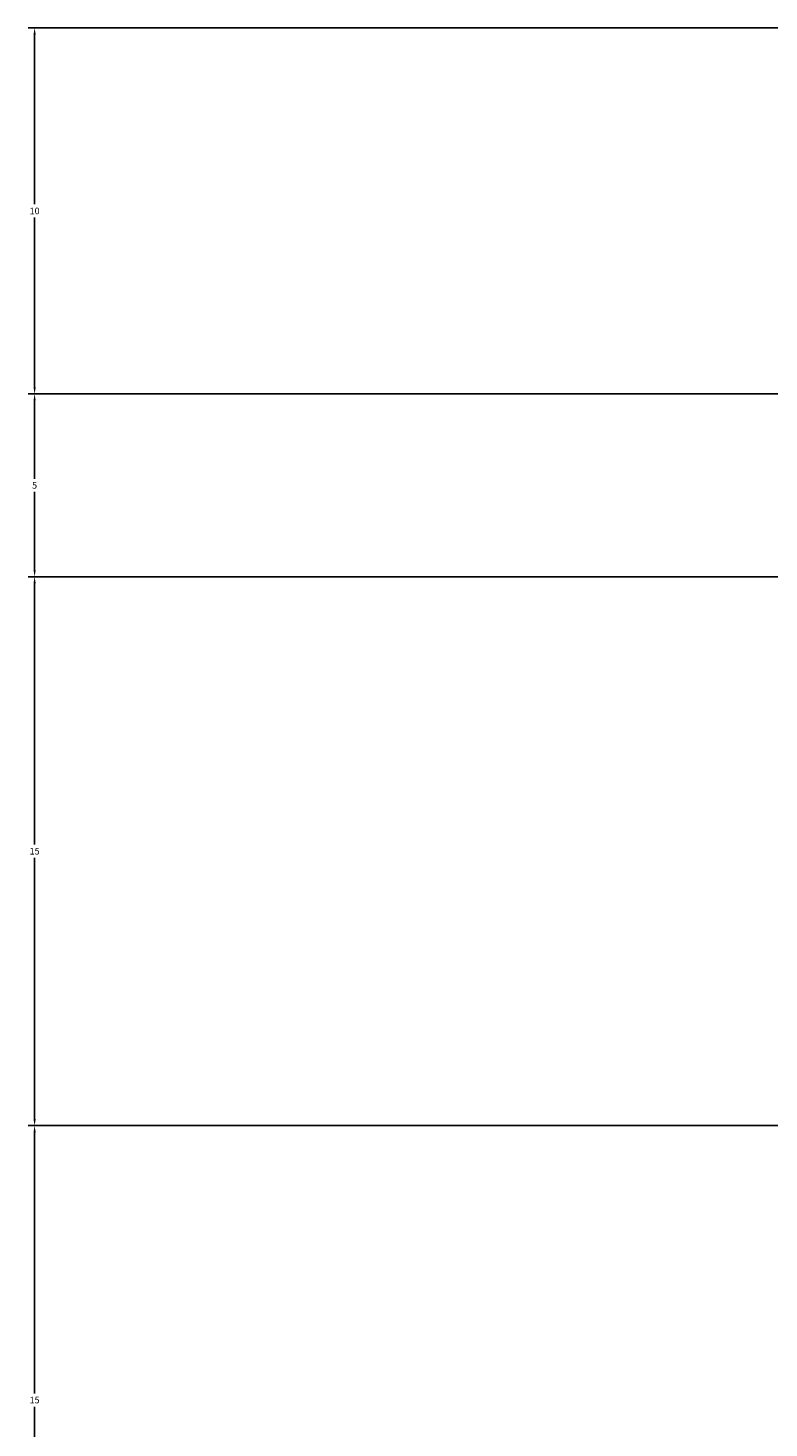
# Model space of a CAD drawing. Units: millimetres. Extents: x -48 to 129, y -118 to -41.
# Tile 2 of 6: x -48 to -28, y -88 to -49. Entities that reach past the tile are written whole.
import ezdxf

# ---------------------------------------------------------------- set-up
doc = ezdxf.new("R2010")
doc.units = ezdxf.units.MM
doc.layers.add('M-DIMS', color=2, linetype='Continuous', lineweight=18)
doc.styles.get("Standard").update_dxf_attribs({"font": 'arial.ttf'})
doc.dimstyles.get("Standard").update_dxf_attribs({"dimtxt": 0.18, "dimasz": 0.18, "dimexe": 0.18, "dimexo": 0.0625, "dimgap": 0.09, "dimtad": 0, "dimtih": 1, "dimtoh": 1, "dimdec": 4, "dimzin": 0, "dimdsep": 46, "dimtxsty": 'Standard', "dimcen": 0.09, "dimadec": 0, "dimazin": 0, "dimtfac": 1, "dimtdec": 4, "dimtofl": 0, "dimtmove": 0, "dimatfit": 3, "dimfxl": 1, "dimtolj": 1, "dimtzin": 0, "dimarcsym": 0})

# ---------------------------------------------------------------- blocks, each defined once
blk = doc.blocks.new('*D1')
at = {"layer": 'Defpoints', "color": 0, "transparency": 16777216}
for p in [(120, -79.442), (-40, -99.442), (120, -117.492)]:
    blk.add_point(p, dxfattribs=at)
at = {"layer": 'M-DIMS', "color": 0, "lineweight": -2, "transparency": 16777216}
for p, q in [((120, -79.505), (120, -117.672)), ((-40, -99.505), (-40, -117.672)), ((-39.82, -117.492), (39.72, -117.492)), ((119.82, -117.492), (40.28, -117.492))]:
    blk.add_line(p, q, dxfattribs=at)
at = {"layer": 'M-DIMS', "color": 0, "transparency": 16777216}
for points in [[(-39.82, -117.462), (-39.82, -117.522), (-40, -117.492)], [(119.82, -117.462), (119.82, -117.522), (120, -117.492)]]:
    blk.add_solid(points, dxfattribs=at)
at = {"layer": 'M-DIMS', "color": 0, "transparency": 16777216, "insert": (40, -117.492), "char_height": 0.18, "attachment_point": 5}
blk.add_mtext('\\A1;160', dxfattribs=at)
blk = doc.blocks.new('*D5')
at = {"layer": 'Defpoints', "color": 0, "transparency": 16777216}
for p in [(-48.05, -79.442), (-20, -79.442), (-40, -94.442)]:
    blk.add_point(p, dxfattribs=at)
at = {"layer": 'M-DIMS', "color": 0, "lineweight": -2, "transparency": 16777216}
for p, q in [((-20.063, -79.442), (-48.23, -79.442)), ((-48.05, -79.622), (-48.05, -86.76)), ((-48.05, -94.262), (-48.05, -87.124)), ((-40.063, -94.442), (-48.23, -94.442))]:
    blk.add_line(p, q, dxfattribs=at)
at = {"layer": 'M-DIMS', "color": 0, "transparency": 16777216}
for points in [[(-48.08, -79.622), (-48.02, -79.622), (-48.05, -79.442)], [(-48.08, -94.262), (-48.02, -94.262), (-48.05, -94.442)]]:
    blk.add_solid(points, dxfattribs=at)
at = {"layer": 'M-DIMS', "color": 0, "transparency": 16777216, "insert": (-48.05, -86.942), "char_height": 0.18, "attachment_point": 5}
blk.add_mtext('\\A1;15', dxfattribs=at)
blk = doc.blocks.new('*D6')
at = {"layer": 'Defpoints', "color": 0, "transparency": 16777216}
for p in [(-48.05, -64.442), (0, -64.442), (-20, -79.442)]:
    blk.add_point(p, dxfattribs=at)
at = {"layer": 'M-DIMS', "color": 0, "lineweight": -2, "transparency": 16777216}
for p, q in [((-0.062, -64.442), (-48.23, -64.442)), ((-48.05, -64.622), (-48.05, -71.76)), ((-48.05, -79.262), (-48.05, -72.124)), ((-20.063, -79.442), (-48.23, -79.442))]:
    blk.add_line(p, q, dxfattribs=at)
at = {"layer": 'M-DIMS', "color": 0, "transparency": 16777216}
for points in [[(-48.08, -64.622), (-48.02, -64.622), (-48.05, -64.442)], [(-48.08, -79.262), (-48.02, -79.262), (-48.05, -79.442)]]:
    blk.add_solid(points, dxfattribs=at)
at = {"layer": 'M-DIMS', "color": 0, "transparency": 16777216, "insert": (-48.05, -71.942), "char_height": 0.18, "attachment_point": 5}
blk.add_mtext('\\A1;15', dxfattribs=at)
blk = doc.blocks.new('*D7')
at = {"layer": 'Defpoints', "color": 0, "transparency": 16777216}
for p in [(-48.05, -59.442), (0, -59.442), (0, -64.442)]:
    blk.add_point(p, dxfattribs=at)
at = {"layer": 'M-DIMS', "color": 0, "lineweight": -2, "transparency": 16777216}
for p, q in [((-0.062, -59.442), (-48.23, -59.442)), ((-48.05, -59.622), (-48.05, -61.761)), ((-48.05, -64.262), (-48.05, -62.124)), ((-0.062, -64.442), (-48.23, -64.442))]:
    blk.add_line(p, q, dxfattribs=at)
at = {"layer": 'M-DIMS', "color": 0, "transparency": 16777216}
for points in [[(-48.08, -59.622), (-48.02, -59.622), (-48.05, -59.442)], [(-48.08, -64.262), (-48.02, -64.262), (-48.05, -64.442)]]:
    blk.add_solid(points, dxfattribs=at)
at = {"layer": 'M-DIMS', "color": 0, "transparency": 16777216, "insert": (-48.05, -61.942), "char_height": 0.18, "attachment_point": 5}
blk.add_mtext('\\A1;5', dxfattribs=at)
blk = doc.blocks.new('*D8')
at = {"layer": 'Defpoints', "color": 0, "transparency": 16777216}
for p in [(-48.05, -49.442), (90, -49.442), (0, -59.442)]:
    blk.add_point(p, dxfattribs=at)
at = {"layer": 'M-DIMS', "color": 0, "lineweight": -2, "transparency": 16777216}
for p, q in [((89.938, -49.442), (-48.23, -49.442)), ((-48.05, -49.622), (-48.05, -54.26)), ((-48.05, -59.262), (-48.05, -54.624)), ((-0.062, -59.442), (-48.23, -59.442))]:
    blk.add_line(p, q, dxfattribs=at)
at = {"layer": 'M-DIMS', "color": 0, "transparency": 16777216}
for points in [[(-48.08, -49.622), (-48.02, -49.622), (-48.05, -49.442)], [(-48.08, -59.262), (-48.02, -59.262), (-48.05, -59.442)]]:
    blk.add_solid(points, dxfattribs=at)
at = {"layer": 'M-DIMS', "color": 0, "transparency": 16777216, "insert": (-48.05, -54.442), "char_height": 0.18, "attachment_point": 5}
blk.add_mtext('\\A1;10', dxfattribs=at)

msp = doc.modelspace()

# ---------------------------------------------------------------- dimensions: what is measured, and where the dimension line sits
at = {"layer": 'M-DIMS'}
for base, p1, p2, picture, middle in [((-48.05, -49.442), (0, -59.442), (90, -49.442), '*D8', (-48.05, -54.442)), ((-48.05, -59.442), (0, -64.442), (0, -59.442), '*D7', (-48.05, -61.942)), ((-48.05, -64.442), (-20, -79.442), (0, -64.442), '*D6', (-48.05, -71.942)), ((-48.05, -79.442), (-40, -94.442), (-20, -79.442), '*D5', (-48.05, -86.942))]:
    dim = msp.add_linear_dim(base=base, p1=p1, p2=p2, angle=90, dimstyle='Standard', override={"dimdec": 0, "dimlfac": 1, "dimrnd": 0, "dimzin": 0, "dimdsep": 46, "dimlunit": 2}, dxfattribs=at)
    dim.commit()
    dim.dimension.update_dxf_attribs({"geometry": picture, "text_midpoint": middle})
dim = msp.add_linear_dim(base=(120, -117.492), p1=(-40, -99.442), p2=(120, -79.442), dimstyle='Standard', override={"dimdec": 0, "dimlfac": 1, "dimrnd": 0, "dimzin": 0, "dimdsep": 46, "dimlunit": 2}, dxfattribs=at)
dim.commit()
dim.dimension.update_dxf_attribs({"geometry": '*D1', "text_midpoint": (40, -117.492)})

doc.saveas('drawing.dxf')
